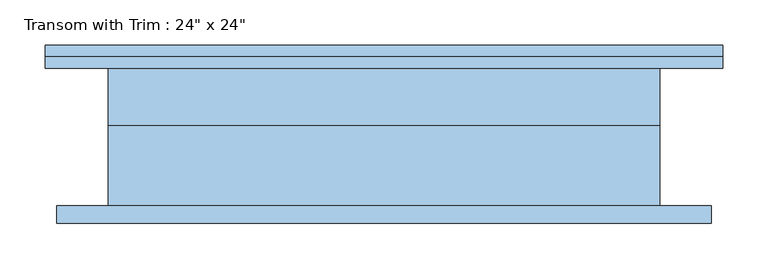
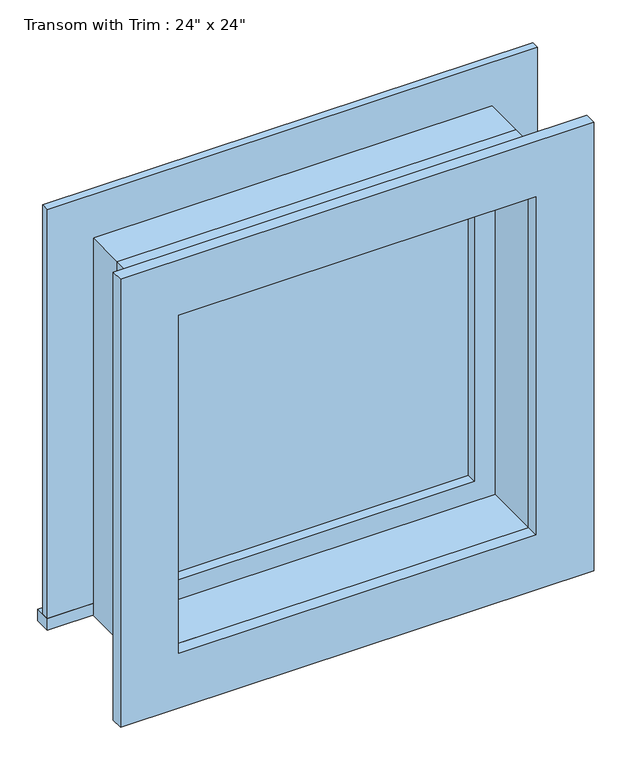
"""IFC4 building model written with IfcOpenShell, lengths in millimetres: window geometry."""

from ifc_helpers import new_model, si_unit, frame, origin, place, context, project, spatial, polyline, outline, extrude, source, transform, mapped, element, save


def window_3d781103(model_context):
    return source(origin(), model_context, "Body", "SweptSolid", [
        extrude(outline(polyline([(-412.75, 101.6), (336.55, 101.6), (336.55, 76.2), (-412.75, 76.2), (-412.75, 101.6)])), frame((0.0, 0.0, 2159.0), z_axis=(0.0, 0.0, 1.0), x_axis=(1.0, 0.0, 0.0)), (0.0, 0.0, 1.0), 19.05),
        extrude(outline(polyline([(2749.55, -323.85), (2749.55, 247.65), (2178.05, 247.65), (2178.05, 336.55), (2838.45, 336.55), (2838.45, -412.75), (2178.05, -412.75), (2178.05, -323.85), (2749.55, -323.85)])), frame((0.0, 76.2, 0.0), z_axis=(0.0, 1.0, 0.0), x_axis=(0.0, 0.0, 1.0)), (0.0, 0.0, 1.0), 12.7),
        extrude(outline(polyline([(2825.75, 323.85), (2825.75, -400.05), (2101.85, -400.05), (2101.85, 323.85), (2825.75, 323.85)]), holes=[polyline([(2736.85, 234.95), (2190.75, 234.95), (2190.75, -311.15), (2736.85, -311.15), (2736.85, 234.95)])]), frame((0.0, -95.25, 0.0), z_axis=(0.0, 1.0, 0.0), x_axis=(0.0, 0.0, 1.0)), (0.0, 0.0, 1.0), 19.05),
        extrude(outline(polyline([(203.2, 28.575), (-279.4, 28.575), (-279.4, 41.275), (203.2, 41.275), (203.2, 28.575)])), frame((0.0, 0.0, 2222.5), z_axis=(0.0, 0.0, 1.0), x_axis=(1.0, 0.0, 0.0)), (0.0, 0.0, 1.0), 482.6),
        extrude(outline(polyline([(2749.55, -323.85), (2178.05, -323.85), (2178.05, 247.65), (2749.55, 247.65), (2749.55, -323.85)]), holes=[polyline([(2705.1, -279.4), (2705.1, 203.2), (2222.5, 203.2), (2222.5, -279.4), (2705.1, -279.4)])]), frame((0.0, 12.7, 0.0), z_axis=(0.0, 1.0, 0.0), x_axis=(0.0, 0.0, 1.0)), (0.0, 0.0, 1.0), 44.45),
        extrude(outline(polyline([(2768.6, -342.9), (2159.0, -342.9), (2159.0, 266.7), (2768.6, 266.7), (2768.6, -342.9)]), holes=[polyline([(2736.85, -311.15), (2736.85, 234.95), (2190.75, 234.95), (2190.75, -311.15), (2736.85, -311.15)])]), frame((0.0, -76.2, 0.0), z_axis=(0.0, 1.0, 0.0), x_axis=(0.0, 0.0, 1.0)), (0.0, 0.0, 1.0), 88.9),
        extrude(outline(polyline([(2768.6, 266.7), (2768.6, -342.9), (2159.0, -342.9), (2159.0, 266.7), (2768.6, 266.7)]), holes=[polyline([(2749.55, 247.65), (2178.05, 247.65), (2178.05, -323.85), (2749.55, -323.85), (2749.55, 247.65)])]), frame((0.0, 12.7, 0.0), z_axis=(0.0, 1.0, 0.0), x_axis=(0.0, 0.0, 1.0)), (0.0, 0.0, 1.0), 63.5),
    ])


if __name__ == "__main__":
    model = new_model("IFC4")
    model_context = context("Model", 3, world=origin())
    ifc_project = project(units=[si_unit("LENGTHUNIT", "METRE", prefix="MILLI")], contexts=[model_context])
    site = spatial("IfcSite", under=ifc_project)
    building = spatial("IfcBuilding", under=site)
    placement = place(None, origin())
    window_shape = window_3d781103(model_context)
    element("IfcWindow", 1, ObjectType="Transom with Trim : 24\" x 24\"", at=placement, inside=building, context=model_context, shape_type="MappedRepresentation", body=[
        mapped(window_shape, transform((0.0, 0.0, 0.0), x_axis=(1.0, 0.0, 0.0), y_axis=(0.0, 1.0, 0.0), z_axis=(0.0, 0.0, 1.0))),
    ])
    save(model, "model.ifc")

# Revit data of these elements
# Type "Transom with Trim : 24\" x 24\""
#   Type Mark = "16"
#   Construction Type Id = "GSP4R"
#   Assembly Code = "B2020100"
#   Analytic Construction = "1/8 in Pilkington single glazing"
#   Visual Light Transmittance = 0.9
#   Solar Heat Gain Coefficient = 0.78
#   Heat Transfer Coefficient (U) = 0.6496 BTU/(h·ft²·°F)
#   Height = 2' - 0"
#   Default Sill Height = 7' - 1"
#   Trim Projection - Ext. = 0' - 0 1/2"
#   Trim Projection - Int. = 0' - 0 3/4"
#   Trim Width - Exterior = 0' - 3 1/2"
#   Trim Width - Interior = 0' - 3 1/2"
#   Width = 2' - 0"
#   Window Inset = 0' - 0 3/4"
#   Define Thermal Properties by = 1
#   Glass Pane Material = Glass
#   Sash Material = Sash
#   Trim Exterior Material = Trim
#   Trim Interior Material = Trim
#   Wall Closure = (empty or 0)
# Element 1 (IfcWindow, "Transom with Trim : 24\" x 24\"")
#   Materials on its faces: "Sash", "Trim", "Glass"
# Materials
#   "Glass": class "Glass", colour RGB 0 128 192, transparency 0.75, Description = "Soda Lime Glass", Cost = 0
#   "Sash": class "Wood", colour RGB 224 178 126, transparency 0
#   "Trim": class "Wood", colour RGB 224 178 126, transparency 0
